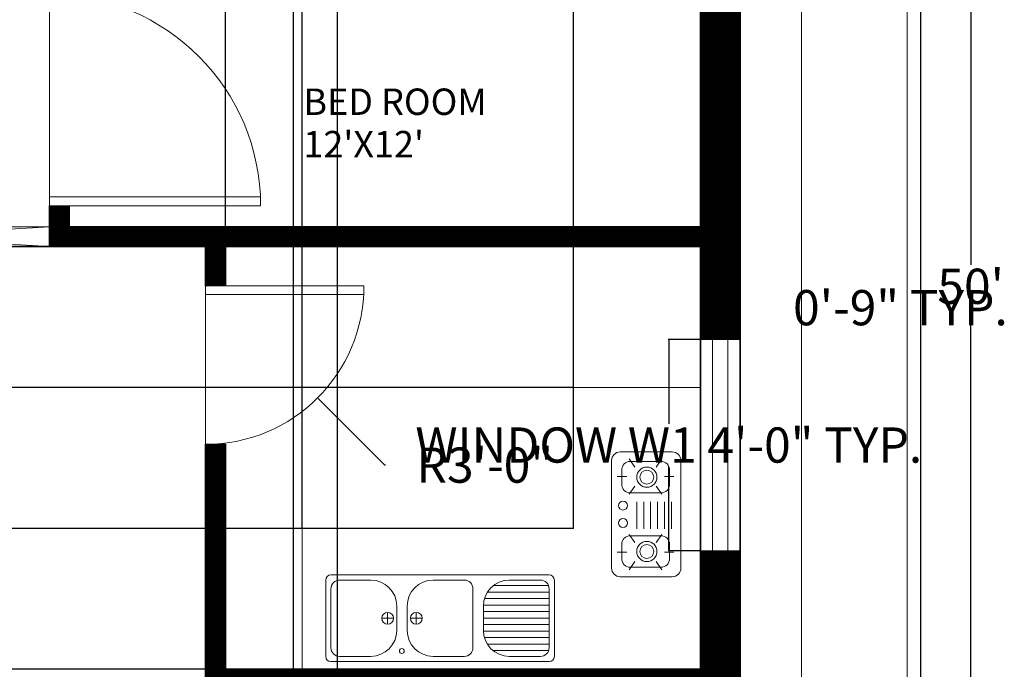
# Model space of a CAD drawing. Units: inches. Extents: x 542 to 1025, y 651 to 1330.
# Tile 3 of 4: x 769 to 993, y 900 to 1048. Entities that reach past the tile are written whole.
import ezdxf

# ---------------------------------------------------------------- set-up
doc = ezdxf.new("R2010")
doc.units = ezdxf.units.IN
doc.header["$MEASUREMENT"] = 0
for name, color, linetype, lineweight in [('A-ANNO-DIMS', 2, 'Continuous', 18), ('A-AREA-IDEN', 7, 'Continuous', 18), ('A-DOOR', 3, 'Continuous', 18), ('A-EQPM', 8, 'Continuous', 18), ('A-FLOR-CASE', 8, 'Continuous', 18), ('A-FLOR-EXTR', 7, 'Continuous', 18), ('A-FLOR-FIXT', 9, 'Continuous', 18), ('A-GLAZ', 4, 'Continuous', 18), ('A-ROOF', 8, 'Continuous', 18), ('A-WALL', 7, 'Continuous', 35), ('A-WALL-OPEN', 4, 'Continuous', 18), ('A-WALL-PATT', 7, 'Continuous', 13), ('C-PROP', 7, 'Continuous', 25)]:
    doc.layers.add(name, color=color, linetype=linetype, lineweight=lineweight)
doc.styles.get("Standard").update_dxf_attribs({"font": 'italic8.shx'})
doc.dimstyles.get("Standard").update_dxf_attribs({"dimtxt": 8, "dimasz": 0.18, "dimexe": 0.18, "dimexo": 0.0625, "dimgap": 0.09, "dimtad": 0, "dimtih": 1, "dimtoh": 1, "dimdec": 4, "dimzin": 0, "dimdsep": 46, "dimlunit": 3, "dimtxsty": 'Standard', "dimcen": 0.09, "dimclrt": 6, "dimadec": 0, "dimazin": 0, "dimtfac": 1, "dimtdec": 4, "dimtofl": 0, "dimtmove": 0, "dimatfit": 3, "dimfxl": 1, "dimtolj": 1, "dimtzin": 0, "dimarcsym": 0})

# ---------------------------------------------------------------- blocks, each defined once
blk = doc.blocks.new('*D4')
at = {"layer": 'A-ANNO-DIMS', "color": 0, "lineweight": -2, "transparency": 16777216}
for p, q in [((974.29, 1287.14), (985.84, 1287.14)), ((985.66, 1286.96), (985.66, 991.99)), ((985.66, 687.32), (985.66, 982.29)), ((974.29, 687.14), (985.84, 687.14))]:
    blk.add_line(p, q, dxfattribs=at)
at = {"layer": 'A-ANNO-DIMS', "color": 0, "transparency": 16777216}
for points in [[(985.63, 1286.96), (985.69, 1286.96), (985.66, 1287.14)], [(985.63, 687.32), (985.69, 687.32), (985.66, 687.14)]]:
    blk.add_solid(points, dxfattribs=at)
at = {"layer": 'Defpoints', "color": 0, "transparency": 16777216}
for p in [(974.23, 1287.14), (974.23, 687.14), (985.66, 687.14)]:
    blk.add_point(p, dxfattribs=at)
at = {"layer": 'A-ANNO-DIMS', "color": 0, "transparency": 16777216, "insert": (985.66, 987.14), "char_height": 8, "attachment_point": 5}
blk.add_mtext("\\A1;50'", dxfattribs=at)
blk = doc.blocks.new('DOOR-SINGLE-48IN')
for p, q in [((48, 0), (48, 48)), ((0, 0), (48, 0)), ((0.04, 2), (48, 2))]:
    blk.add_line(p, q)
blk.add_arc((48, 0), 48, 90, 180)
blk = doc.blocks.new('WINDOW-48IN')
for p, q in [((0, 48), (0, 0)), ((9, 48), (0, 48)), ((0, 48), (4.5, 48)), ((2.75, 48), (2.75, 0)), ((6.25, 48), (6.25, 0)), ((9, 0), (9, 48)), ((0, 0), (9, 0))]:
    blk.add_line(p, q)
blk = doc.blocks.new('*D12')
at = {"layer": 'A-ANNO-DIMS', "color": 0, "lineweight": -2, "transparency": 16777216}
for p, q in [((924.17, 975.08), (916.85, 975.08)), ((917.03, 974.9), (917.03, 955.93)), ((917.03, 927.26), (917.03, 946.22)), ((924.17, 927.08), (916.85, 927.08))]:
    blk.add_line(p, q, dxfattribs=at)
at = {"layer": 'A-ANNO-DIMS', "color": 0, "transparency": 16777216}
for points in [[(917, 974.9), (917.06, 974.9), (917.03, 975.08)], [(917, 927.26), (917.06, 927.26), (917.03, 927.08)]]:
    blk.add_solid(points, dxfattribs=at)
at = {"layer": 'Defpoints', "color": 0, "transparency": 16777216}
for p in [(917.03, 975.08), (924.23, 975.08), (924.23, 927.08)]:
    blk.add_point(p, dxfattribs=at)
at = {"layer": 'A-ANNO-DIMS', "color": 6, "transparency": 16777216, "insert": (917.03, 951.08), "char_height": 8, "attachment_point": 5}
blk.add_mtext('\\A1;WINDOW W1 4\'-0" TYP.', dxfattribs=at)
blk = doc.blocks.new('*D13')
at = {"layer": 'A-ANNO-DIMS', "color": 0, "lineweight": -2, "transparency": 16777216}
for p, q in [((924.23, 975.14), (924.23, 982.46)), ((924.41, 982.28), (933.05, 982.28)), ((933.23, 975.14), (933.23, 982.46)), ((933.23, 982.28), (933.41, 982.28))]:
    blk.add_line(p, q, dxfattribs=at)
at = {"layer": 'A-ANNO-DIMS', "color": 0, "transparency": 16777216}
for points in [[(924.41, 982.31), (924.41, 982.25), (924.23, 982.28)], [(933.05, 982.31), (933.05, 982.25), (933.23, 982.28)]]:
    blk.add_solid(points, dxfattribs=at)
at = {"layer": 'Defpoints', "color": 0, "transparency": 16777216}
for p in [(933.23, 982.28), (924.23, 975.08), (933.23, 975.08)]:
    blk.add_point(p, dxfattribs=at)
at = {"layer": 'A-ANNO-DIMS', "color": 6, "transparency": 16777216, "insert": (969.69, 982.28), "char_height": 8, "attachment_point": 5}
blk.add_mtext('\\A1;0\'-9" TYP.', dxfattribs=at)
blk = doc.blocks.new('*D26')
at = {"layer": 'A-ANNO-DIMS', "color": 0, "lineweight": -2, "transparency": 16777216}
for p, q in [((816.23, 996.2), (816.23, 1318.37)), ((816.41, 1318.19), (852.23, 1318.19)), ((924.05, 1318.19), (888.22, 1318.19)), ((924.23, 996.2), (924.23, 1318.37))]:
    blk.add_line(p, q, dxfattribs=at)
at = {"layer": 'A-ANNO-DIMS', "color": 0, "transparency": 16777216}
for points in [[(816.41, 1318.22), (816.41, 1318.16), (816.23, 1318.19)], [(924.05, 1318.22), (924.05, 1318.16), (924.23, 1318.19)]]:
    blk.add_solid(points, dxfattribs=at)
at = {"layer": 'Defpoints', "color": 0, "transparency": 16777216}
for p in [(924.23, 1318.19), (816.23, 996.14), (924.23, 996.14)]:
    blk.add_point(p, dxfattribs=at)
at = {"layer": 'A-ANNO-DIMS', "color": 6, "transparency": 16777216, "insert": (870.23, 1318.19), "char_height": 8, "attachment_point": 5}
blk.add_mtext('\\A1;9\'-0"', dxfattribs=at)
blk = doc.blocks.new('*D27')
at = {"layer": 'A-ANNO-DIMS', "color": 0, "lineweight": -2, "transparency": 16777216}
for p, q in [((816.17, 996.14), (583, 996.14)), ((583.18, 995.96), (583.18, 952.99)), ((583.18, 900.32), (583.18, 943.29)), ((816.17, 900.14), (583, 900.14))]:
    blk.add_line(p, q, dxfattribs=at)
at = {"layer": 'A-ANNO-DIMS', "color": 0, "transparency": 16777216}
for points in [[(583.15, 995.96), (583.21, 995.96), (583.18, 996.14)], [(583.15, 900.32), (583.21, 900.32), (583.18, 900.14)]]:
    blk.add_solid(points, dxfattribs=at)
at = {"layer": 'Defpoints', "color": 0, "transparency": 16777216}
for p in [(583.18, 996.14), (816.23, 996.14), (816.23, 900.14)]:
    blk.add_point(p, dxfattribs=at)
at = {"layer": 'A-ANNO-DIMS', "color": 6, "transparency": 16777216, "insert": (583.18, 948.14), "char_height": 8, "attachment_point": 5}
blk.add_mtext('\\A1;8\'-0"', dxfattribs=at)
blk = doc.blocks.new('*D30')
at = {"layer": 'A-ANNO-DIMS', "color": 0, "lineweight": -2, "transparency": 16777216}
for p, q in [((831.73, 811.7), (831.73, 1318.37)), ((831.91, 1318.19), (841.55, 1318.19)), ((841.73, 811.7), (841.73, 1318.37)), ((841.73, 1318.19), (841.91, 1318.19))]:
    blk.add_line(p, q, dxfattribs=at)
at = {"layer": 'A-ANNO-DIMS', "color": 0, "transparency": 16777216}
for points in [[(831.91, 1318.22), (831.91, 1318.16), (831.73, 1318.19)], [(841.55, 1318.22), (841.55, 1318.16), (841.73, 1318.19)]]:
    blk.add_solid(points, dxfattribs=at)
at = {"layer": 'Defpoints', "color": 0, "transparency": 16777216}
for p in [(841.73, 1318.19), (831.73, 811.64), (841.73, 811.64)]:
    blk.add_point(p, dxfattribs=at)
at = {"layer": 'A-ANNO-DIMS', "color": 6, "transparency": 16777216, "insert": (862.57, 1318.19), "char_height": 8, "attachment_point": 5}
blk.add_mtext('\\A1;0\'-10"', dxfattribs=at)
blk = doc.blocks.new('*D31')
at = {"layer": 'A-ANNO-DIMS', "color": 0, "lineweight": -2, "transparency": 16777216}
for p, q in [((833.7, 932.22), (833.7, 1318.37)), ((833.88, 1318.19), (895.2, 1318.19)), ((895.38, 932.22), (895.38, 1318.37)), ((895.38, 1318.19), (895.56, 1318.19))]:
    blk.add_line(p, q, dxfattribs=at)
at = {"layer": 'A-ANNO-DIMS', "color": 0, "transparency": 16777216}
for points in [[(833.88, 1318.22), (833.88, 1318.16), (833.7, 1318.19)], [(895.2, 1318.22), (895.2, 1318.16), (895.38, 1318.19)]]:
    blk.add_solid(points, dxfattribs=at)
at = {"layer": 'Defpoints', "color": 0, "transparency": 16777216}
for p in [(895.38, 1318.19), (833.7, 932.16), (895.38, 932.16)]:
    blk.add_point(p, dxfattribs=at)
at = {"layer": 'A-ANNO-DIMS', "color": 6, "transparency": 16777216, "insert": (927.46, 1318.19), "char_height": 8, "attachment_point": 5}
blk.add_mtext('\\A1;5\'-1 1/2"', dxfattribs=at)
blk = doc.blocks.new('*D32')
at = {"layer": 'A-ANNO-DIMS', "color": 0, "lineweight": -2, "transparency": 16777216}
for p, q in [((895.32, 964.12), (583, 964.12)), ((583.18, 963.94), (583.18, 952.99)), ((583.18, 932.34), (583.18, 943.29)), ((895.32, 932.16), (583, 932.16))]:
    blk.add_line(p, q, dxfattribs=at)
at = {"layer": 'A-ANNO-DIMS', "color": 0, "transparency": 16777216}
for points in [[(583.15, 963.94), (583.21, 963.94), (583.18, 964.12)], [(583.15, 932.34), (583.21, 932.34), (583.18, 932.16)]]:
    blk.add_solid(points, dxfattribs=at)
at = {"layer": 'Defpoints', "color": 0, "transparency": 16777216}
for p in [(583.18, 964.12), (895.38, 964.12), (895.38, 932.16)]:
    blk.add_point(p, dxfattribs=at)
at = {"layer": 'A-ANNO-DIMS', "color": 6, "transparency": 16777216, "insert": (583.18, 948.14), "char_height": 8, "attachment_point": 5}
blk.add_mtext('\\A1;2\'-8"', dxfattribs=at)
blk = doc.blocks.new('*D33')
at = {"layer": 'A-ANNO-DIMS', "color": 0, "lineweight": -2, "transparency": 16777216}
for p, q in [((833.64, 932.16), (583, 932.16)), ((583.18, 931.98), (583.18, 921)), ((583.18, 900.32), (583.18, 911.3)), ((833.64, 900.14), (583, 900.14))]:
    blk.add_line(p, q, dxfattribs=at)
at = {"layer": 'A-ANNO-DIMS', "color": 0, "transparency": 16777216}
for points in [[(583.15, 931.98), (583.21, 931.98), (583.18, 932.16)], [(583.15, 900.32), (583.21, 900.32), (583.18, 900.14)]]:
    blk.add_solid(points, dxfattribs=at)
at = {"layer": 'Defpoints', "color": 0, "transparency": 16777216}
for p in [(583.18, 932.16), (833.7, 932.16), (833.7, 900.14)]:
    blk.add_point(p, dxfattribs=at)
at = {"layer": 'A-ANNO-DIMS', "color": 6, "transparency": 16777216, "insert": (583.18, 916.15), "char_height": 8, "attachment_point": 5}
blk.add_mtext('\\A1;2\'-8"', dxfattribs=at)
blk = doc.blocks.new('*D34')
at = {"layer": 'A-ANNO-DIMS', "color": 0, "lineweight": -2, "transparency": 16777216}
for p, q in [((895.38, 964.19), (895.38, 1318.37)), ((895.56, 1318.19), (924.05, 1318.19)), ((924.23, 964.19), (924.23, 1318.37)), ((924.23, 1318.19), (924.41, 1318.19))]:
    blk.add_line(p, q, dxfattribs=at)
at = {"layer": 'A-ANNO-DIMS', "color": 0, "transparency": 16777216}
for points in [[(895.56, 1318.22), (895.56, 1318.16), (895.38, 1318.19)], [(924.05, 1318.22), (924.05, 1318.16), (924.23, 1318.19)]]:
    blk.add_solid(points, dxfattribs=at)
at = {"layer": 'Defpoints', "color": 0, "transparency": 16777216}
for p in [(924.23, 1318.19), (895.38, 964.12), (924.23, 964.12)]:
    blk.add_point(p, dxfattribs=at)
at = {"layer": 'A-ANNO-DIMS', "color": 6, "transparency": 16777216, "insert": (942.4, 1318.19), "char_height": 8, "attachment_point": 5}
blk.add_mtext('\\A1;2\'-5"', dxfattribs=at)
blk = doc.blocks.new('*D35')
at = {"layer": 'A-ANNO-DIMS', "color": 0, "lineweight": -2, "transparency": 16777216}
for p, q in [((811.64, 987.25), (811.82, 987.25)), ((811.73, 987.16), (811.73, 987.34)), ((852.46, 946.52), (837.31, 961.66)), ((852.64, 946.52), (852.46, 946.52))]:
    blk.add_line(p, q, dxfattribs=at)
at = {"layer": 'A-ANNO-DIMS', "color": 0, "transparency": 16777216}
blk.add_solid([(837.33, 961.69), (837.29, 961.64), (837.18, 961.79)], dxfattribs=at)
at = {"layer": 'Defpoints', "color": 0, "transparency": 16777216}
for p in [(811.73, 987.25), (837.18, 961.79)]:
    blk.add_point(p, dxfattribs=at)
at = {"layer": 'A-ANNO-DIMS', "color": 6, "transparency": 16777216, "insert": (875.2, 946.52), "char_height": 8, "attachment_point": 5}
blk.add_mtext('\\A1;R3\'-0"', dxfattribs=at)

msp = doc.modelspace()

# ---------------------------------------------------------------- hatches: boundary and pattern name
at = {"layer": 'A-WALL-PATT'}
h = msp.add_hatch(dxfattribs=at)
h.set_pattern_fill('ANSI31', color=256)
h.set_pattern_definition([(45, (-552.11989, -271.07657), (-0.088388348, 0.088388348), [])])
h.paths.add_polyline_path([(715.041, 1218.14134), (623.2294, 1218.14134), (623.2294, 1278.14134), (687.2294, 1278.14134), (687.2294, 1287.14134), (614.2294, 1287.14134), (614.2294, 1150.81788), (618.7294, 1150.81788), (623.2294, 1150.81788), (623.2294, 1209.14134), (715.041, 1209.14134)])
h.paths.add_polyline_path([(864.47291, 1213.64134), (864.47291, 1218.14134), (763.041, 1218.14134), (763.041, 1213.64134), (763.041, 1209.14134), (776.2294, 1209.14134), (776.2294, 1065.14134), (769.45548, 1065.14134), (769.45548, 1060.64134), (776.2294, 1060.64134), (776.2294, 1053.42968), (780.7294, 1053.42968), (780.7294, 1144.64134), (780.7294, 1209.14134), (840.2294, 1209.14134), (840.2294, 1181.73273), (844.7294, 1181.73273), (844.7294, 1209.14134), (864.47291, 1209.14134)])
h.paths.add_polyline_path([(933.2294, 1218.14134), (894.47291, 1218.14134), (894.47291, 1209.14134), (924.2294, 1209.14134), (924.2294, 1144.64134), (924.2294, 1100.56821), (928.7294, 1100.56821), (933.2294, 1100.56821)])
h.paths.add_polyline_path([(933.2294, 1052.56821), (924.2294, 1052.56821), (924.2294, 1000.64134), (780.7294, 1000.64134), (780.7294, 1005.42968), (776.2294, 1005.42968), (776.2294, 996.14134), (780.7294, 996.14134), (811.7294, 996.14134), (811.7294, 987.24818), (816.2294, 987.24818), (816.2294, 996.14134), (924.2294, 996.14134), (924.2294, 975.07641), (928.7294, 975.07641), (933.2294, 975.07641)])
h.paths.add_polyline_path([(924.2294, 1149.14134), (844.7294, 1149.14134), (844.7294, 1151.73273), (840.2294, 1151.73273), (840.2294, 1149.14134), (831.41283, 1149.14134), (831.41283, 1144.64134), (924.2294, 1144.64134)])
h.paths.add_polyline_path([(623.2294, 1102.81788), (614.2294, 1102.81788), (614.2294, 1047.96339), (618.7294, 1047.96339), (623.2294, 1047.96339), (623.2294, 1060.64134), (655.18423, 1060.64134), (655.18423, 1065.14134), (623.2294, 1065.14134)])
h.paths.add_polyline_path([(721.45548, 1065.14134), (685.18423, 1065.14134), (685.18423, 1060.64134), (695.2294, 1060.64134), (695.2294, 1000.64134), (623.2294, 1000.64134), (623.2294, 1017.96339), (614.2294, 1017.96339), (614.2294, 996.14134), (666.7294, 996.14134), (666.7294, 976.55402), (671.2294, 976.55402), (675.7294, 976.55402), (675.7294, 996.14134), (699.7294, 996.14134), (699.7294, 1060.64134), (721.45548, 1060.64134)])
h.paths.add_polyline_path([(675.7294, 928.55402), (666.7294, 928.55402), (666.7294, 904.64134), (614.2294, 904.64134), (614.2294, 879.38817), (618.7294, 879.38817), (623.2294, 879.38817), (623.2294, 900.14134), (671.2294, 900.14134), (671.2294, 828.14134), (666.89138, 828.14134), (666.89138, 819.14134), (743.2294, 819.14134), (743.2294, 754.70501), (752.2294, 754.70501), (752.2294, 802.64134), (753.36467, 802.64134), (753.36467, 811.64134), (752.2294, 811.64134), (752.2294, 828.14134), (675.7294, 828.14134)])
h.paths.add_polyline_path([(636.89138, 828.14134), (623.2294, 828.14134), (623.2294, 849.38817), (614.2294, 849.38817), (614.2294, 778.30684), (618.7294, 778.30684), (623.2294, 778.30684), (623.2294, 819.14134), (636.89138, 819.14134)], flags=17)
h.paths.add_polyline_path([(864.47291, 811.64134), (847.39014, 811.64134), (847.39014, 802.64134), (864.47291, 802.64134)], flags=17)
h.paths.add_polyline_path([(817.39014, 811.64134), (807.36467, 811.64134), (807.36467, 802.64134), (817.39014, 802.64134), (817.39014, 807.14134)])
h.paths.add_polyline_path([(933.2294, 927.07641), (924.2294, 927.07641), (924.2294, 900.14134), (816.2294, 900.14134), (816.2294, 951.24818), (811.7294, 951.24818), (811.7294, 895.64134), (928.7294, 895.64134), (928.7294, 811.64134), (894.47291, 811.64134), (894.47291, 802.64134), (933.2294, 802.64134)])
h.paths.add_polyline_path([(752.2294, 706.70501), (743.2294, 706.70501), (743.2294, 696.14134), (712.47774, 696.14134), (712.47774, 691.64134), (712.47774, 687.14134), (752.2294, 687.14134)])
h.paths.add_polyline_path([(664.47774, 696.14134), (623.2294, 696.14134), (623.2294, 730.30684), (614.2294, 730.30684), (614.2294, 687.14134), (664.47774, 687.14134)])
h.paths.add_polyline_path([(925.1985, 1143.73295), (966.26993, 1143.73295), (966.26993, 1152.66152), (925.1985, 1152.66152)], flags=9)
h.paths.add_polyline_path([(925.4366, 1152.0031), (965.31755, 1152.0031), (965.31755, 1159.5031), (925.4366, 1159.5031)], flags=9)

# ---------------------------------------------------------------- linework, layer by layer
at = {"layer": 'A-DOOR'}
for p, q in [((780.7294, 1005.42968), (776.2294, 1005.42968)), ((811.7294, 987.24818), (816.2294, 987.24818)), ((847.7294, 987.24818), (811.7294, 987.24818)), ((811.7294, 987.24818), (811.7294, 951.24818)), ((847.6738, 985.24818), (811.7294, 985.24818)), ((811.7294, 951.24818), (816.2294, 951.24818))]:
    msp.add_line(p, q, dxfattribs=at)
msp.add_arc((811.7294, 987.24818), 36, 270, 0, dxfattribs=at)
at = {"layer": 'A-EQPM'}
for p, q in [((905.99802, 949.51575), (917.80902, 949.51575)), ((904.02952, 923.13785), (904.02952, 947.54725)), ((908.03864, 947.93846), (909.32728, 946.07438)), ((915.23383, 947.3649), (908.28894, 947.3649)), ((915.48414, 947.93846), (914.1955, 946.07438)), ((919.77752, 947.54725), (919.77752, 923.13785)), ((906.32044, 945.3964), (906.32044, 942.16387)), ((917.20233, 942.16387), (917.20233, 945.3964)), ((905.31817, 943.92352), (907.46591, 943.92352)), ((918.20461, 943.92352), (916.05687, 943.92352)), ((908.03864, 939.90859), (909.32728, 941.77266)), ((908.28894, 940.19537), (915.23383, 940.19537)), ((915.48414, 939.90859), (914.1955, 941.77266)), ((909.75788, 938.1879), (909.75788, 932.0221)), ((911.33268, 938.1879), (911.33268, 932.0221)), ((912.90748, 938.1879), (912.90748, 932.0221)), ((914.48228, 938.1879), (914.48228, 932.0221)), ((916.05708, 938.1879), (916.05708, 932.0221)), ((917.63188, 938.1879), (917.63188, 932.0221)), ((908.03864, 930.77652), (909.32728, 928.91245)), ((908.28894, 930.48974), (915.23383, 930.48974)), ((915.48414, 930.77652), (914.1955, 928.91245)), ((905.31817, 926.76159), (907.46591, 926.76159)), ((906.32044, 925.28871), (906.32044, 928.52124)), ((918.20461, 926.76159), (916.05687, 926.76159)), ((917.20233, 928.52124), (917.20233, 925.28871)), ((908.03864, 922.74665), (909.32728, 924.61073)), ((915.48414, 922.74665), (914.1955, 924.61073)), ((915.23383, 923.32021), (908.28894, 923.32021)), ((917.80902, 921.16935), (905.99802, 921.16935))]:
    msp.add_line(p, q, dxfattribs=at)
for centre, radius in [((912.04775, 943.78013), 2.29425), ((912.04775, 943.78013), 1.5773), ((906.60681, 937.32756), 1.00373), ((906.60681, 933.35755), 1.00373), ((912.04775, 926.90498), 2.29425), ((912.04775, 926.90498), 1.5773)]:
    msp.add_circle(centre, radius, dxfattribs=at)
for centre, start, end in [((905.99802, 947.54725), 90, 180), ((917.80902, 947.54725), 0, 90), ((908.28894, 945.3964), 90, 180), ((915.23383, 945.3964), 0, 90), ((908.28894, 942.16387), 180, 270), ((915.23383, 942.16387), 270, 0), ((908.28894, 928.52124), 90, 180), ((915.23383, 928.52124), 0, 90), ((908.28894, 925.28871), 180, 270), ((915.23383, 925.28871), 270, 0), ((905.99802, 923.13785), 180, 270), ((917.80902, 923.13785), 270, 0)]:
    msp.add_arc(centre, 1.9685, start, end, dxfattribs=at)
at = {"layer": 'A-FLOR-CASE'}
for p, q in [((924.2294, 964.12283), (895.38156, 964.12283)), ((895.38156, 964.12283), (895.38156, 932.15804)), ((895.38156, 932.15804), (833.70082, 932.15804)), ((833.70082, 932.15804), (833.70082, 900.14134))]:
    msp.add_line(p, q, dxfattribs=at)
at = {"layer": 'A-FLOR-EXTR'}
msp.add_line((971.2294, 1284.14134), (971.2294, 802.5643), dxfattribs=at)
at = {"layer": 'A-FLOR-FIXT'}
for p, q in [((839.04026, 903.07586), (839.04026, 920.39866)), ((889.82756, 921.57976), (840.22136, 921.57976)), ((849.27646, 920.39866), (842.18986, 920.39866)), ((863.44966, 920.39866), (870.53626, 920.39866)), ((880.77246, 920.39866), (887.85906, 920.39866)), ((891.00866, 903.07586), (891.00866, 920.39866)), ((840.22136, 905.04436), (840.22136, 918.43016)), ((872.50476, 905.04436), (872.50476, 918.43016)), ((889.6883, 919.137), (877.14654, 919.137)), ((889.82756, 905.04436), (889.82756, 918.43016)), ((889.82756, 916.18425), (875.12005, 916.18425)), ((889.82756, 917.66062), (875.79972, 917.66062)), ((855.18196, 908.98136), (855.18196, 914.49316)), ((857.54416, 908.98136), (857.54416, 914.49316)), ((874.86696, 908.98136), (874.86696, 914.49316)), ((889.82756, 914.70787), (874.8723, 914.70787)), ((851.77022, 911.73726), (854.45282, 911.73726)), ((853.11152, 910.39597), (853.11152, 913.07856)), ((858.27331, 911.73726), (860.95591, 911.73726)), ((859.61461, 910.39597), (859.61461, 913.07856)), ((889.82756, 913.2315), (874.86696, 913.2315)), ((889.82756, 911.75512), (874.86696, 911.75512)), ((889.82756, 910.27875), (874.86696, 910.27875)), ((889.82756, 908.80237), (874.86845, 908.80237)), ((889.82756, 907.326), (875.09817, 907.326)), ((889.82756, 905.84962), (875.75463, 905.84962)), ((889.71677, 904.37325), (877.0576, 904.37325)), ((849.27646, 903.07586), (842.18986, 903.07586)), ((863.44966, 903.07586), (870.53626, 903.07586)), ((880.77246, 903.07586), (887.85906, 903.07586)), ((889.82756, 901.89476), (840.22136, 901.89476))]:
    msp.add_line(p, q, dxfattribs=at)
for centre, radius in [((853.11152, 911.73726), 1.3413), ((859.61461, 911.73726), 1.3413), ((856.34145, 904.2874), 0.5539)]:
    msp.add_circle(centre, radius, dxfattribs=at)
for centre, radius, start, end in [((840.22136, 920.39866), 1.1811, 90, 180), ((842.18986, 918.43016), 1.9685, 90, 180), ((849.27646, 914.49316), 5.9055, 0, 90), ((863.44966, 914.49316), 5.9055, 90, 180), ((870.53626, 918.43016), 1.9685, 360, 90), ((880.77246, 914.49316), 5.9055, 90, 180), ((887.85906, 918.43016), 1.9685, 360, 90), ((889.82756, 920.39866), 1.1811, 0, 90), ((849.27646, 908.98136), 5.9055, 270, 0), ((863.44966, 908.98136), 5.9055, 180, 270), ((880.77246, 908.98136), 5.9055, 180, 270), ((842.18986, 905.04436), 1.9685, 180, 270), ((870.53626, 905.04436), 1.9685, 270, 360), ((887.85906, 905.04436), 1.9685, 270, 360), ((840.22136, 903.07586), 1.1811, 180, 270), ((889.82756, 903.07586), 1.1811, 270, 0)]:
    msp.add_arc(centre, radius, start, end, dxfattribs=at)
at = {"layer": 'A-ROOF'}
msp.add_line((947.2294, 1236.14134), (947.2294, 802.5643), dxfattribs=at)
at = {"layer": 'A-WALL'}
for p, q in [((933.2294, 1218.14134), (933.2294, 802.64134)), ((924.2294, 1144.64134), (924.2294, 1000.64134)), ((776.2294, 996.14134), (776.2294, 1005.42968)), ((780.7294, 1000.64134), (780.7294, 1005.42968)), ((780.7294, 1000.64134), (924.2294, 1000.64134)), ((675.7294, 996.14134), (780.7294, 996.14134)), ((780.7294, 996.14134), (811.7294, 996.14134)), ((811.7294, 996.14134), (811.7294, 987.24818)), ((816.2294, 996.14134), (816.2294, 987.24818)), ((816.2294, 996.14134), (924.2294, 996.14134)), ((924.2294, 996.14134), (924.2294, 900.14134)), ((811.7294, 951.24818), (811.7294, 895.64134)), ((816.2294, 951.24818), (816.2294, 900.14134)), ((816.2294, 900.14134), (924.2294, 900.14134))]:
    msp.add_line(p, q, dxfattribs=at)
at = {"layer": 'A-WALL-OPEN'}
for p, q in [((699.7294, 1000.64134), (776.2294, 1000.64134)), ((699.7294, 996.14134), (776.2294, 1000.64134)), ((776.2294, 996.14134), (699.7294, 1000.64134)), ((776.2294, 1000.64134), (776.2294, 996.14134))]:
    msp.add_line(p, q, dxfattribs=at)
at = {"layer": 'C-PROP'}
msp.add_line((974.2294, 1287.14134), (974.2294, 687.14134), dxfattribs=at)

# ---------------------------------------------------------------- block references
at = {"layer": 'A-DOOR', "extrusion": (0, 0, -1), "zscale": -1}
msp.add_blockref('DOOR-SINGLE-48IN', (-824.2298, 1005.42967), dxfattribs=at)
at = {"layer": 'A-GLAZ'}
msp.add_blockref('WINDOW-48IN', (924.229, 927.0762), dxfattribs=at)

# ---------------------------------------------------------------- texts
at = {"layer": 'A-AREA-IDEN'}
for s, p in [('BED ROOM', (833.9496, 1026.06301)), ("12'X12'", (833.9496, 1016.42454))]:
    msp.add_text(s, height=6, dxfattribs=at).set_placement(p)

# ---------------------------------------------------------------- dimensions: what is measured, and where the dimension line sits
at = {"layer": 'A-ANNO-DIMS'}
for base, p1, p2, picture, middle in [((895.38156, 1318.19134), (833.70082, 932.15804), (895.38156, 932.15804), '*D31', (927.46108, 1318.19134)), ((924.2294, 1318.19134), (816.2294, 996.14134), (924.2294, 996.14134), '*D26', (870.2294, 1318.19134)), ((841.7294, 1318.19134), (831.7294, 811.64134), (841.7294, 811.64134), '*D30', (862.57083, 1318.19134)), ((924.2294, 1318.19134), (895.38156, 964.12283), (924.2294, 964.12283), '*D34', (942.40416, 1318.19134))]:
    dim = msp.add_linear_dim(base=base, p1=p1, p2=p2, dimstyle='Standard', override={"dimdec": 1, "dimlfac": 1, "dimrnd": 0, "dimzin": 1, "dimdsep": 46, "dimlunit": 4, "dimfrac": 2}, dxfattribs=at)
    dim.commit()
    dim.dimension.update_dxf_attribs({"geometry": picture, "text_midpoint": middle})
for base, p1, p2, override, picture, middle in [((985.65631, 687.14134), (974.2294, 1287.14134), (974.2294, 687.14134), {"dimclrd": 0, "dimclre": 0, "dimclrt": 0}, '*D4', (985.65631, 987.14134)), ((583.1794, 996.14134), (816.2294, 900.14134), (816.2294, 996.14134), {"dimdec": 1, "dimlfac": 1, "dimrnd": 0, "dimzin": 1, "dimdsep": 46, "dimlunit": 4, "dimfrac": 2}, '*D27', (583.1794, 948.14134)), ((583.1794, 964.12283), (895.38156, 932.15804), (895.38156, 964.12283), {"dimdec": 1, "dimlfac": 1, "dimrnd": 0, "dimzin": 1, "dimdsep": 46, "dimlunit": 4, "dimfrac": 2}, '*D32', (583.1794, 948.14044)), ((583.1794, 932.15804), (833.70082, 900.14134), (833.70082, 932.15804), {"dimdec": 1, "dimlfac": 1, "dimrnd": 0, "dimzin": 1, "dimdsep": 46, "dimlunit": 4, "dimfrac": 2}, '*D33', (583.1794, 916.14969))]:
    dim = msp.add_linear_dim(base=base, p1=p1, p2=p2, angle=90, dimstyle='Standard', override=override, dxfattribs=at)
    dim.commit()
    dim.dimension.update_dxf_attribs({"geometry": picture, "text_midpoint": middle})
dim = msp.add_linear_dim(base=(933.2294, 982.27641), p1=(924.2294, 975.07641), p2=(933.2294, 975.07641), text='<> TYP.', dimstyle='Standard', override={"dimdec": 1, "dimlfac": 1, "dimrnd": 0, "dimzin": 1, "dimdsep": 46, "dimlunit": 4, "dimfrac": 2}, dxfattribs=at)
dim.commit()
dim.dimension.update_dxf_attribs({"geometry": '*D13', "text_midpoint": (969.68988, 982.27641)})
dim = msp.add_radius_dim(center=(811.7294, 987.24818), mpoint=(837.18495, 961.79205), dimstyle='Standard', override={"dimdec": 1, "dimlfac": 1, "dimrnd": 0, "dimzin": 1, "dimdsep": 46, "dimlunit": 4, "dimfrac": 2}, dxfattribs=at)
dim.commit()
dim.dimension.update_dxf_attribs({"geometry": '*D35', "text_midpoint": (875.20447, 946.51837), "dimtype": 164})
dim = msp.add_linear_dim(base=(917.0294, 975.07641), p1=(924.2294, 927.07641), p2=(924.2294, 975.07641), angle=90, text='WINDOW W1 <> TYP.', dimstyle='Standard', override={"dimdec": 1, "dimlfac": 1, "dimrnd": 0, "dimzin": 1, "dimdsep": 46, "dimlunit": 4, "dimfrac": 2}, dxfattribs=at)
dim.commit()
dim.dimension.update_dxf_attribs({"geometry": '*D12', "text_midpoint": (917.0294, 951.07641)})

doc.saveas('drawing.dxf')
